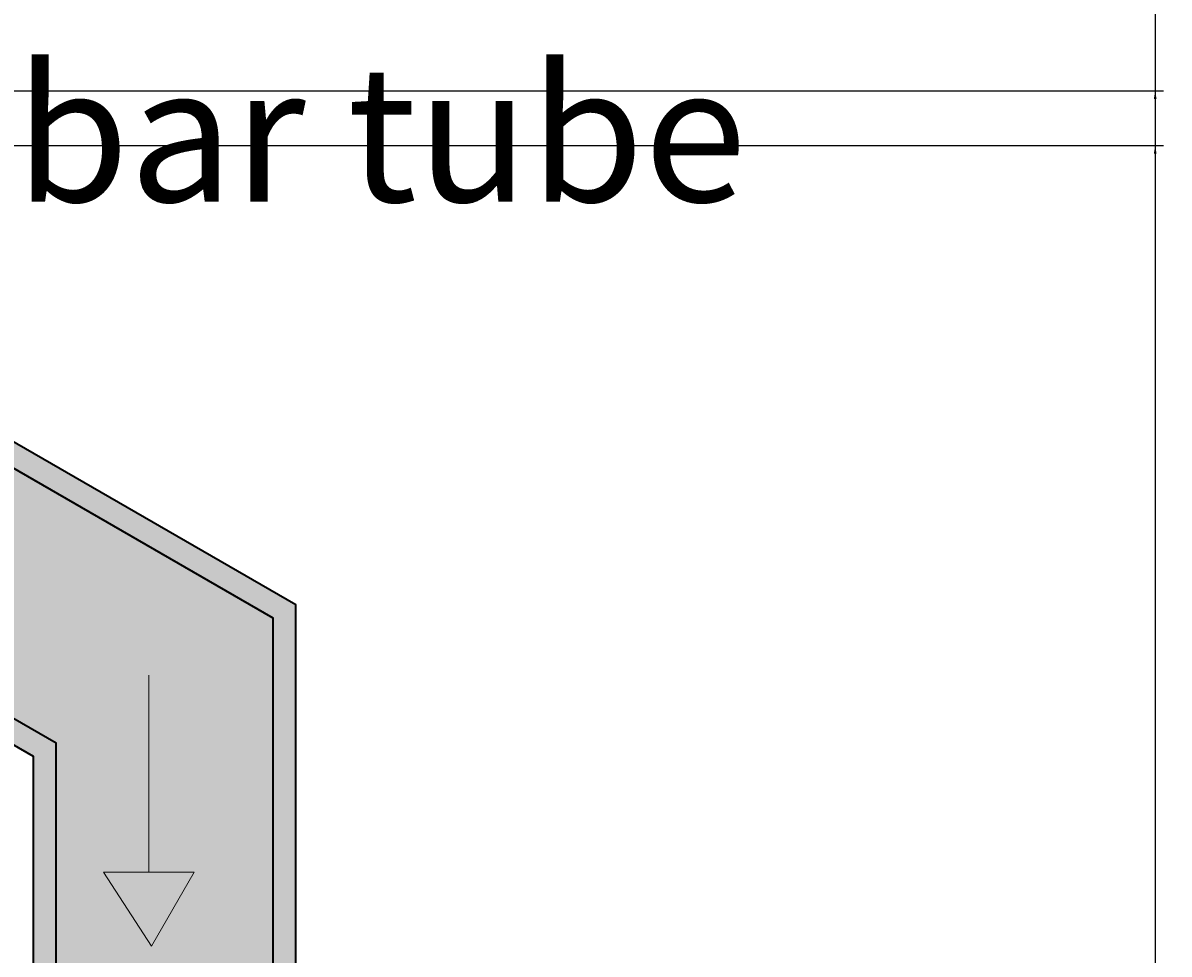
# Model space of a CAD drawing. Units: inches. Extents: x -1 to 292, y -3 to 199.
# Tile 50 of 52: x 267 to 292, y 81 to 101. Entities that reach past the tile are written whole.
import ezdxf

# ---------------------------------------------------------------- set-up
doc = ezdxf.new("R2010")
doc.units = ezdxf.units.IN
doc.header["$MEASUREMENT"] = 0
for name, color, linetype, lineweight in [('M-ANNO-SYMB', 1, 'Continuous', 18), ('M-ANNO-TEXT', 3, 'Continuous', 25), ('M-DIMS', 2, 'Continuous', 18), ('M-EQPM', 7, 'Continuous', 35), ('M-PATT', 8, 'Continuous', 13)]:
    doc.layers.add(name, color=color, linetype=linetype, lineweight=lineweight)
doc.styles.get("Standard").update_dxf_attribs({"font": 'arial.ttf'})
doc.dimstyles.get("Standard").update_dxf_attribs({"dimtxt": 0.18, "dimasz": 0.18, "dimexe": 0.18, "dimexo": 0.0625, "dimgap": 0.09, "dimtad": 0, "dimtih": 1, "dimtoh": 1, "dimdec": 4, "dimzin": 0, "dimdsep": 46, "dimtxsty": 'Standard', "dimcen": 0.09, "dimadec": 0, "dimazin": 0, "dimtfac": 1, "dimtdec": 4, "dimtofl": 0, "dimtmove": 0, "dimatfit": 3, "dimfxl": 1, "dimtolj": 1, "dimtzin": 0, "dimarcsym": 0})

# ---------------------------------------------------------------- blocks, each defined once
blk = doc.blocks.new('FLOW-ARROW-WATER')
blk.add_line((223.29, 53.741), (227.063, 51.564))
blk.add_lwpolyline([(222.79, 52.875), (221.849, 54.506), (223.79, 54.608)], close=True)
blk = doc.blocks.new('*D10')
at = {"layer": 'Defpoints', "color": 0, "transparency": 16777216}
for p in [(169.176, 99.774), (169.176, 43.391), (292.04, 43.391)]:
    blk.add_point(p, dxfattribs=at)
at = {"layer": 'M-DIMS', "color": 0, "lineweight": -2, "transparency": 16777216}
for p, q in [((169.239, 99.774), (292.22, 99.774)), ((292.04, 99.594), (292.04, 71.764)), ((292.04, 43.571), (292.04, 71.4)), ((169.239, 43.391), (292.22, 43.391))]:
    blk.add_line(p, q, dxfattribs=at)
at = {"layer": 'M-DIMS', "color": 0, "transparency": 16777216}
for points in [[(292.01, 99.594), (292.07, 99.594), (292.04, 99.774)], [(292.01, 43.571), (292.07, 43.571), (292.04, 43.391)]]:
    blk.add_solid(points, dxfattribs=at)
at = {"layer": 'M-DIMS', "color": 0, "transparency": 16777216, "insert": (292.04, 71.582), "char_height": 0.18, "attachment_point": 5}
blk.add_mtext('\\A1;56.38', dxfattribs=at)
blk = doc.blocks.new('*D25')
at = {"layer": 'Defpoints', "color": 0, "transparency": 16777216}
for p in [(273.066, 88.419), (215.241, 88.13), (273.066, -2.71)]:
    blk.add_point(p, dxfattribs=at)
at = {"layer": 'M-DIMS', "color": 0, "lineweight": -2, "transparency": 16777216}
for p, q in [((273.066, 88.357), (273.066, -2.89)), ((215.241, 88.068), (215.241, -2.89)), ((215.421, -2.71), (243.76, -2.71)), ((272.886, -2.71), (244.547, -2.71))]:
    blk.add_line(p, q, dxfattribs=at)
at = {"layer": 'M-DIMS', "color": 0, "transparency": 16777216}
for points in [[(215.421, -2.68), (215.421, -2.74), (215.241, -2.71)], [(272.886, -2.68), (272.886, -2.74), (273.066, -2.71)]]:
    blk.add_solid(points, dxfattribs=at)
at = {"layer": 'M-DIMS', "color": 0, "transparency": 16777216, "insert": (244.153, -2.71), "char_height": 0.18, "attachment_point": 5}
blk.add_mtext('\\A1;57.83', dxfattribs=at)
blk = doc.blocks.new('*D29')
at = {"layer": 'Defpoints', "color": 0, "transparency": 16777216}
for p in [(243.903, 98.567), (243.903, 44.598), (292.04, 44.598)]:
    blk.add_point(p, dxfattribs=at)
at = {"layer": 'M-DIMS', "color": 0, "lineweight": -2, "transparency": 16777216}
for p, q in [((243.966, 98.567), (292.22, 98.567)), ((292.04, 98.387), (292.04, 71.764)), ((292.04, 44.778), (292.04, 71.4)), ((243.966, 44.598), (292.22, 44.598))]:
    blk.add_line(p, q, dxfattribs=at)
at = {"layer": 'M-DIMS', "color": 0, "transparency": 16777216}
for points in [[(292.01, 98.387), (292.07, 98.387), (292.04, 98.567)], [(292.01, 44.778), (292.07, 44.778), (292.04, 44.598)]]:
    blk.add_solid(points, dxfattribs=at)
at = {"layer": 'M-DIMS', "color": 0, "transparency": 16777216, "insert": (292.04, 71.582), "char_height": 0.18, "attachment_point": 5}
blk.add_mtext('\\A1;53.97', dxfattribs=at)
blk = doc.blocks.new('*D33')
at = {"layer": 'Defpoints', "color": 0, "transparency": 16777216}
for p in [(242.955, 125.727), (292.04, 125.727), (237.933, 30.73)]:
    blk.add_point(p, dxfattribs=at)
at = {"layer": 'M-DIMS', "color": 0, "lineweight": -2, "transparency": 16777216}
for p, q in [((243.018, 125.727), (292.22, 125.727)), ((292.04, 125.547), (292.04, 78.41)), ((292.04, 30.91), (292.04, 78.046)), ((237.996, 30.73), (292.22, 30.73))]:
    blk.add_line(p, q, dxfattribs=at)
at = {"layer": 'M-DIMS', "color": 0, "transparency": 16777216}
for points in [[(292.01, 125.547), (292.07, 125.547), (292.04, 125.727)], [(292.01, 30.91), (292.07, 30.91), (292.04, 30.73)]]:
    blk.add_solid(points, dxfattribs=at)
at = {"layer": 'M-DIMS', "color": 0, "transparency": 16777216, "insert": (292.04, 78.228), "char_height": 0.18, "attachment_point": 5}
blk.add_mtext('\\A1;95', dxfattribs=at)

msp = doc.modelspace()

# ---------------------------------------------------------------- hatches: boundary and pattern name
at = {"layer": 'M-PATT'}
h = msp.add_hatch(color=256, dxfattribs=at)
h.set_gradient(color1=(0, 255, 255), color2=(0, 255, 255), tint=1, name='CYLINDER')
h.paths.add_polyline_path([(256.8092, 99.5764), (256.4077, 99.3157), (253.7155, 100.87), (251.3221, 99.3157), (248.6299, 100.87), (246.2365, 99.3157), (243.5443, 100.87), (241.1509, 99.3157), (238.4587, 100.87), (236.4209, 99.5466), (236.4209, 97.1861), (234.9209, 97.1861), (234.9209, 99.9764), (233.3731, 100.87), (230.9797, 99.3157, 1.0704128)])
h.paths.add_polyline_path([(234.4549, 44.5975, 1), (253.3518, 44.5975, 1)])
h.paths.add_polyline_path([(235.4822, 48.8821), (220.034, 57.8011), (220.034, 85.363), (232.4507, 92.5318, -0.0853739), (231.0925, 96.7051), (215.7407, 87.8418), (215.7407, 55.3224), (234.4552, 44.5176, -0.0021162), (234.4549, 44.5975, -0.1182098)])
h.paths.add_polyline_path([(222.7904, 52.8755), (221.8492, 54.5058), (223.7904, 54.6075)], flags=16)
h.paths.add_polyline_path([(216.828, 66.8912), (217.7692, 68.5216), (218.828, 66.8912)], flags=16)
h.paths.add_polyline_path([(216.8084, 83.826), (217.7497, 85.4564), (218.8084, 83.826)], flags=16)
h.paths.add_polyline_path([(226.468, 92.8803), (228.3442, 93.0348), (227.6068, 91.2362)], flags=16)
h.paths.add_polyline_path([(272.5659, 88.1304), (260.2765, 95.2257), (259.0113, 93.0196), (263.0639, 91.1046), (263.4912, 92.0087), (264.5631, 90.4612), (262.6367, 90.2004), (263.0639, 91.1046), (259.0113, 93.0196), (257.8918, 91.0677), (267.7726, 85.363), (267.7726, 57.8011), (255.5043, 50.718), (257.0663, 46.085), (272.5659, 55.0337)])
h.paths.add_polyline_path([(263.6286, 51.5636), (261.7461, 51.5636), (262.6286, 53.2956)], flags=16)
h.paths.add_polyline_path([(269.8773, 65.3608), (268.8186, 66.9911), (270.8186, 66.9911)], flags=16)
h.paths.add_polyline_path([(269.8773, 80.8843), (268.8186, 82.5146), (270.8186, 82.5146)], flags=16)
h.paths.add_polyline_path([(255.5043, 50.718), (252.3244, 48.8821, -0.1182098), (253.3518, 44.5975, -0.0177685), (253.3279, 43.9266), (257.0663, 46.085)])
h.paths.add_polyline_path([(260.2765, 95.2257), (256.7809, 97.2439, -0.0959457), (255.356, 92.5318), (257.8918, 91.0677)])
h = msp.add_hatch(color=256, dxfattribs=at)
h.set_gradient(color1=(76, 38, 47), color2=(76, 38, 47), tint=1, name='CYLINDER')
h.paths.add_polyline_path([(267.2726, 58.0898), (255.3414, 51.2013), (255.5043, 50.718), (267.7726, 57.8011), (267.7726, 85.363), (257.8918, 91.0677), (257.643, 90.634), (267.2726, 85.0743)])
h.paths.add_polyline_path([(272.5659, 55.0337), (257.0663, 46.085), (257.2293, 45.6017), (273.0659, 54.745), (273.0659, 88.4191), (260.5253, 95.6595), (260.2765, 95.2257), (272.5659, 88.1304)])
h.paths.add_polyline_path([(215.2407, 55.0337), (234.4787, 43.9266, -0.0156517), (234.4552, 44.5176), (215.7407, 55.3224), (215.7407, 87.8418), (231.0925, 96.7051, -0.0104859), (231.0257, 97.2439), (215.2407, 88.1304)])
h.paths.add_polyline_path([(220.034, 57.8011), (235.4822, 48.8821, -0.0132367), (235.7207, 49.3218), (220.534, 58.0898), (220.534, 85.0743), (232.6923, 92.0939, -0.0096587), (232.4507, 92.5318), (220.034, 85.363)])
h = msp.add_hatch(color=256, dxfattribs=at)
h.set_gradient(color1=(0, 0, 255), color2=(0, 0, 255), tint=1, name='CYLINDER')
h.paths.add_polyline_path([(227.6068, 91.2362), (228.3442, 93.0348), (226.468, 92.8803)])
h.paths.add_polyline_path([(218.8084, 83.826), (217.7497, 85.4564), (216.8084, 83.826)])
h.paths.add_polyline_path([(262.6367, 90.2004), (264.5631, 90.4612), (263.4912, 92.0087)])
h.paths.add_polyline_path([(217.7692, 68.5216), (216.828, 66.8912), (218.828, 66.8912)])
h.paths.add_polyline_path([(223.7904, 54.6075), (221.8492, 54.5058), (222.7904, 52.8755)])
h.paths.add_polyline_path([(262.6286, 53.2956), (261.7461, 51.5636), (263.6286, 51.5636)])
h.paths.add_polyline_path([(268.8186, 82.5146), (269.8773, 80.8843), (270.8186, 82.5146)])
h.paths.add_polyline_path([(268.8186, 66.9911), (269.8773, 65.3608), (270.8186, 66.9911)])

# ---------------------------------------------------------------- linework, layer by layer
at = {"layer": 'M-EQPM'}
for points in [[(253.2639, 43.3124), (273.0659, 54.745), (273.0659, 88.4191), (256.8257, 97.7954)], [(253.3279, 43.9266), (272.5659, 55.0337), (272.5659, 88.1304), (256.7809, 97.2439)], [(252.3359, 48.8887), (267.7726, 57.8011), (267.7726, 85.363), (255.356, 92.5318)], [(252.0859, 49.3218), (267.2726, 58.0898), (267.2726, 85.0743), (255.1143, 92.0939)]]:
    msp.add_lwpolyline(points, dxfattribs=at)

# ---------------------------------------------------------------- block references
at = {"layer": 'M-ANNO-SYMB', "rotation": 120.0000000000007}
msp.add_blockref('FLOW-ARROW-WATER', (428.0053, -83.9899), dxfattribs=at)

# ---------------------------------------------------------------- texts
at = {"layer": 'M-ANNO-TEXT', "insert": (266.8556, 100.3254), "char_height": 3, "attachment_point": 1}
msp.add_mtext_dynamic_manual_height_columns('bar tube', width=23.906137, gutter_width=1, heights=[0], dxfattribs=at)

# ---------------------------------------------------------------- dimensions: what is measured, and where the dimension line sits
at = {"layer": 'M-DIMS'}
for base, p1, p2, override, picture, middle in [((292.0399, 125.7269), (237.9333, 30.7296), (242.9552, 125.7269), {"dimdec": 0, "dimlfac": 1, "dimrnd": 0, "dimzin": 0, "dimdsep": 46, "dimlunit": 2}, '*D33', (292.0399, 78.2282)), ((292.0399, 43.3906), (169.176, 99.7735), (169.176, 43.3906), {"dimdec": 2, "dimlfac": 1, "dimrnd": 0, "dimzin": 0, "dimdsep": 46, "dimlunit": 2}, '*D10', (292.0399, 71.5821)), ((292.0399, 44.5975), (243.9033, 98.5666), (243.9033, 44.5975), {"dimdec": 2, "dimlfac": 1, "dimrnd": 0, "dimzin": 0, "dimdsep": 46, "dimlunit": 2}, '*D29', (292.0399, 71.5821))]:
    dim = msp.add_linear_dim(base=base, p1=p1, p2=p2, angle=90, dimstyle='Standard', override=override, dxfattribs=at)
    dim.commit()
    dim.dimension.update_dxf_attribs({"geometry": picture, "text_midpoint": middle})
dim = msp.add_linear_dim(base=(273.0659, -2.7104), p1=(215.2407, 88.1304), p2=(273.0659, 88.4191), dimstyle='Standard', override={"dimdec": 2, "dimlfac": 1, "dimrnd": 0, "dimzin": 0, "dimdsep": 46, "dimlunit": 2}, dxfattribs=at)
dim.commit()
dim.dimension.update_dxf_attribs({"geometry": '*D25', "text_midpoint": (244.1533, -2.7104)})

doc.saveas('drawing.dxf')
